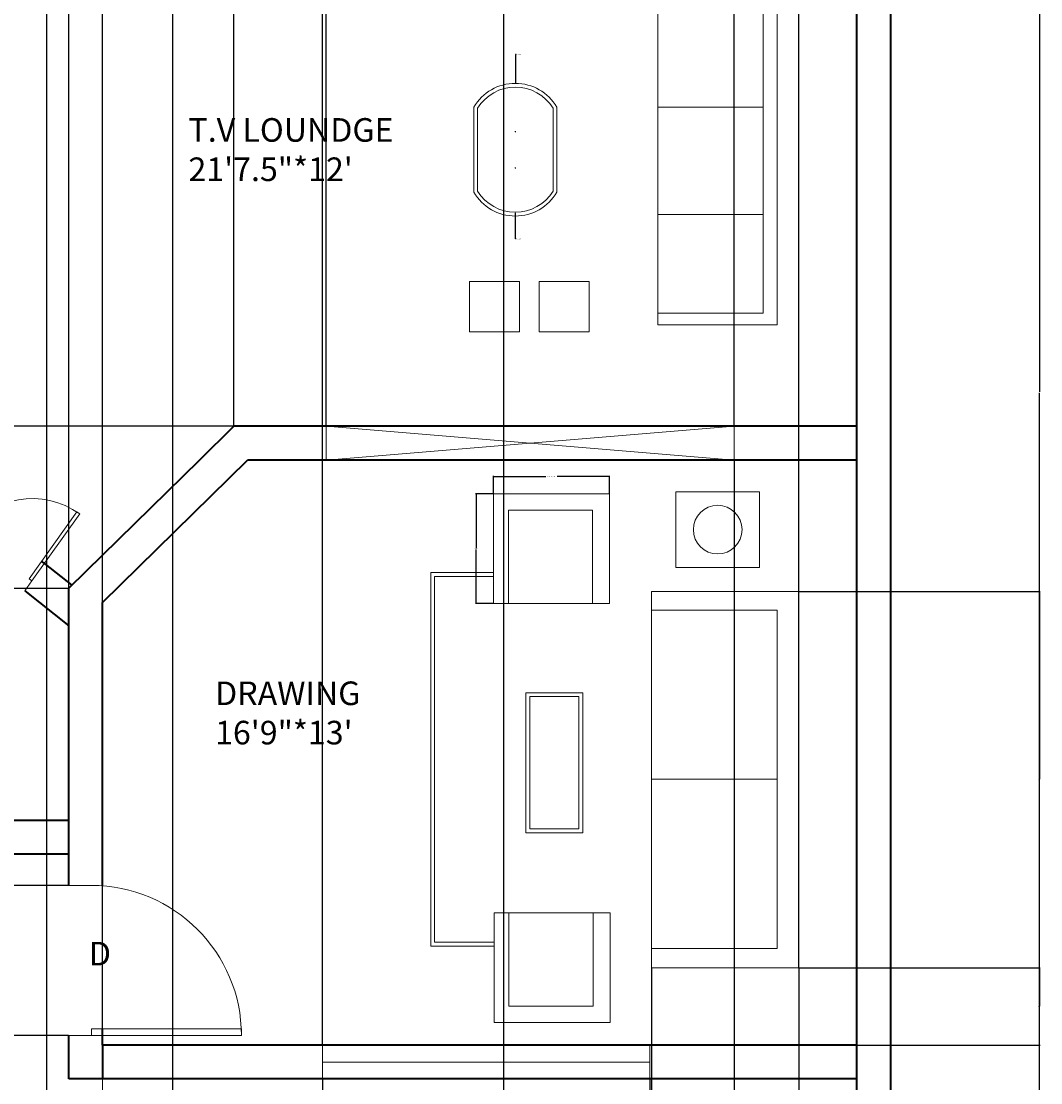
# Model space of a CAD drawing. Units: inches. Extents: x 2284 to 2815, y 1123 to 1948.
# Tile 4 of 6: x 2543 to 2815, y 1358 to 1641. Entities that reach past the tile are written whole.
import ezdxf

# ---------------------------------------------------------------- set-up
doc = ezdxf.new("R2010")
doc.units = ezdxf.units.IN
for name, color, linetype, lineweight in [('A-ANNO-DIMS', 2, 'Continuous', 18), ('A-AREA-IDEN', 30, 'Continuous', 18), ('A-WALL-PATT', 140, 'Continuous', 13), ('C-SITE-PVMT', 7, 'Continuous', 18), ('C-SITE-WALL', 7, 'Continuous', 35), ('DOOR', 190, 'Continuous', 18), ('FUR', 10, 'Continuous', 18), ('TEXT', 30, 'Continuous', 18), ('WALL', 7, 'Continuous', 35), ('WIND', 210, 'Continuous', 18)]:
    doc.layers.add(name, color=color, linetype=linetype, lineweight=lineweight)
doc.styles.get("Standard").update_dxf_attribs({"font": 'arial.ttf'})
doc.dimstyles.get("Standard").update_dxf_attribs({"dimtxt": 0.18, "dimasz": 0.18, "dimexe": 0.18, "dimexo": 0.0625, "dimgap": 0.09, "dimtad": 0, "dimtih": 1, "dimtoh": 1, "dimdec": 4, "dimzin": 0, "dimdsep": 46, "dimtxsty": 'Standard', "dimcen": 0.09, "dimadec": 0, "dimazin": 0, "dimtfac": 1, "dimtdec": 4, "dimtofl": 0, "dimtmove": 0, "dimatfit": 3, "dimfxl": 1, "dimtolj": 1, "dimtzin": 0, "dimarcsym": 0})

# ---------------------------------------------------------------- blocks, each defined once
blk = doc.blocks.new('*U2')
for p, q in [((0, 0), (0, -6)), ((40, 0), (40, -6))]:
    blk.add_line(p, q)
blk.add_lwpolyline([(0, 0), (0, 40), (1.75, 40), (1.75, 0)], close=True)
blk.add_arc((0, 0), 40, 0, 90)
blk = doc.blocks.new('LOUNGE-CHAIR')
for p, q in [((3.98, 0), (3.98, 24.94)), ((3.98, 24.94), (26.41, 24.94)), ((26.41, 24.94), (26.41, 0))]:
    blk.add_line(p, q)
blk.add_lwpolyline([(30.95, 0), (0, 0), (0, 29.22), (30.95, 29.22)], close=True)
blk = doc.blocks.new('*D18')
at = {"layer": 'A-ANNO-DIMS', "color": 0, "lineweight": -2, "transparency": 16777216}
for p, q in [((2668.74, 1515.42), (2668.74, 1520.18)), ((2668.92, 1520), (2682.69, 1520)), ((2699.5, 1520), (2685.73, 1520)), ((2699.68, 1515.42), (2699.68, 1520.18))]:
    blk.add_line(p, q, dxfattribs=at)
at = {"layer": 'A-ANNO-DIMS', "color": 0, "transparency": 16777216}
for points in [[(2668.92, 1520.03), (2668.92, 1519.97), (2668.74, 1520)], [(2699.5, 1520.03), (2699.5, 1519.97), (2699.68, 1520)]]:
    blk.add_solid(points, dxfattribs=at)
at = {"layer": 'Defpoints', "color": 0, "transparency": 16777216}
for p in [(2699.68, 1520), (2668.74, 1515.36), (2699.68, 1515.36)]:
    blk.add_point(p, dxfattribs=at)
at = {"layer": 'A-ANNO-DIMS', "color": 0, "transparency": 16777216, "insert": (2684.21, 1520), "char_height": 0.18, "attachment_point": 5}
blk.add_mtext('\\A1;LOUNGE CHAIR 31 TYP.', dxfattribs=at)
blk = doc.blocks.new('*D19')
at = {"layer": 'A-ANNO-DIMS', "color": 0, "lineweight": -2, "transparency": 16777216}
for p, q in [((2668.67, 1515.36), (2663.91, 1515.36)), ((2664.09, 1515.18), (2664.09, 1500.93)), ((2664.09, 1486.32), (2664.09, 1500.57)), ((2668.67, 1486.14), (2663.91, 1486.14))]:
    blk.add_line(p, q, dxfattribs=at)
at = {"layer": 'A-ANNO-DIMS', "color": 0, "transparency": 16777216}
for points in [[(2664.06, 1515.18), (2664.12, 1515.18), (2664.09, 1515.36)], [(2664.06, 1486.32), (2664.12, 1486.32), (2664.09, 1486.14)]]:
    blk.add_solid(points, dxfattribs=at)
at = {"layer": 'Defpoints', "color": 0, "transparency": 16777216}
for p in [(2664.09, 1515.36), (2668.74, 1515.36), (2668.74, 1486.14)]:
    blk.add_point(p, dxfattribs=at)
at = {"layer": 'A-ANNO-DIMS', "color": 0, "transparency": 16777216, "insert": (2664.09, 1500.75), "char_height": 0.18, "attachment_point": 5}
blk.add_mtext('\\A1;29 TYP.', dxfattribs=at)
blk = doc.blocks.new('*D21')
at = {"layer": 'A-ANNO-DIMS', "color": 0, "lineweight": -2, "transparency": 16777216}
for p, q in [((2774.62, 1908.4), (2814.43, 1908.4)), ((2814.25, 1908.22), (2814.25, 1542.59)), ((2814.25, 1176.58), (2814.25, 1542.22)), ((2774.62, 1176.4), (2814.43, 1176.4))]:
    blk.add_line(p, q, dxfattribs=at)
at = {"layer": 'A-ANNO-DIMS', "color": 0, "transparency": 16777216}
for points in [[(2814.22, 1908.22), (2814.28, 1908.22), (2814.25, 1908.4)], [(2814.22, 1176.58), (2814.28, 1176.58), (2814.25, 1176.4)]]:
    blk.add_solid(points, dxfattribs=at)
at = {"layer": 'Defpoints', "color": 0, "transparency": 16777216}
for p in [(2774.55, 1908.4), (2814.25, 1908.4), (2774.55, 1176.4)]:
    blk.add_point(p, dxfattribs=at)
at = {"layer": 'A-ANNO-DIMS', "color": 0, "transparency": 16777216, "insert": (2814.25, 1542.4), "char_height": 0.18, "attachment_point": 5}
blk.add_mtext('\\A1;732', dxfattribs=at)
blk = doc.blocks.new('*D42')
at = {"layer": 'A-ANNO-DIMS', "color": 0, "lineweight": -2, "transparency": 16777216}
for p, q in [((2623.18, 1359.34), (2623.18, 1136.52)), ((2710.41, 1359.34), (2710.41, 1136.52)), ((2623.36, 1136.7), (2666.4, 1136.7)), ((2710.23, 1136.7), (2667.19, 1136.7))]:
    blk.add_line(p, q, dxfattribs=at)
at = {"layer": 'A-ANNO-DIMS', "color": 0, "transparency": 16777216}
for points in [[(2623.36, 1136.73), (2623.36, 1136.67), (2623.18, 1136.7)], [(2710.23, 1136.73), (2710.23, 1136.67), (2710.41, 1136.7)]]:
    blk.add_solid(points, dxfattribs=at)
at = {"layer": 'Defpoints', "color": 0, "transparency": 16777216}
for p in [(2623.18, 1359.4), (2710.41, 1359.4), (2710.41, 1136.7)]:
    blk.add_point(p, dxfattribs=at)
at = {"layer": 'A-ANNO-DIMS', "color": 0, "transparency": 16777216, "insert": (2666.79, 1136.7), "char_height": 0.18, "attachment_point": 5}
blk.add_mtext('\\A1;87.23', dxfattribs=at)
blk = doc.blocks.new('*D43')
at = {"layer": 'A-ANNO-DIMS', "color": 0, "lineweight": -2, "transparency": 16777216}
for p, q in [((2564.55, 1368.47), (2564.55, 1948.28)), ((2564.73, 1948.1), (2593.47, 1948.1)), ((2623, 1948.1), (2594.26, 1948.1)), ((2623.18, 1368.47), (2623.18, 1948.28))]:
    blk.add_line(p, q, dxfattribs=at)
at = {"layer": 'A-ANNO-DIMS', "color": 0, "transparency": 16777216}
for points in [[(2564.73, 1948.13), (2564.73, 1948.07), (2564.55, 1948.1)], [(2623, 1948.13), (2623, 1948.07), (2623.18, 1948.1)]]:
    blk.add_solid(points, dxfattribs=at)
at = {"layer": 'Defpoints', "color": 0, "transparency": 16777216}
for p in [(2623.18, 1948.1), (2564.55, 1368.4), (2623.18, 1368.4)]:
    blk.add_point(p, dxfattribs=at)
at = {"layer": 'A-ANNO-DIMS', "color": 0, "transparency": 16777216, "insert": (2593.87, 1948.1), "char_height": 0.18, "attachment_point": 5}
blk.add_mtext('\\A1;58.62', dxfattribs=at)
blk = doc.blocks.new('*D44')
at = {"layer": 'A-ANNO-DIMS', "color": 0, "lineweight": -2, "transparency": 16777216}
for p, q in [((2583.19, 1836.34), (2583.19, 1136.52)), ((2671.4, 1836.34), (2671.4, 1136.52)), ((2583.37, 1136.7), (2626.92, 1136.7)), ((2671.22, 1136.7), (2627.67, 1136.7))]:
    blk.add_line(p, q, dxfattribs=at)
at = {"layer": 'A-ANNO-DIMS', "color": 0, "transparency": 16777216}
for points in [[(2583.37, 1136.73), (2583.37, 1136.67), (2583.19, 1136.7)], [(2671.22, 1136.73), (2671.22, 1136.67), (2671.4, 1136.7)]]:
    blk.add_solid(points, dxfattribs=at)
at = {"layer": 'Defpoints', "color": 0, "transparency": 16777216}
for p in [(2583.19, 1836.4), (2671.4, 1836.4), (2671.4, 1136.7)]:
    blk.add_point(p, dxfattribs=at)
at = {"layer": 'A-ANNO-DIMS', "color": 0, "transparency": 16777216, "insert": (2627.29, 1136.7), "char_height": 0.18, "attachment_point": 5}
blk.add_mtext('\\A1;88.21', dxfattribs=at)
blk = doc.blocks.new('*D45')
at = {"layer": 'A-ANNO-DIMS', "color": 0, "lineweight": -2, "transparency": 16777216}
for p, q in [((2549.55, 1836.34), (2549.55, 1136.52)), ((2583.19, 1836.34), (2583.19, 1136.52)), ((2549.73, 1136.7), (2565.91, 1136.7)), ((2583.01, 1136.7), (2566.84, 1136.7))]:
    blk.add_line(p, q, dxfattribs=at)
at = {"layer": 'A-ANNO-DIMS', "color": 0, "transparency": 16777216}
for points in [[(2549.73, 1136.73), (2549.73, 1136.67), (2549.55, 1136.7)], [(2583.01, 1136.73), (2583.01, 1136.67), (2583.19, 1136.7)]]:
    blk.add_solid(points, dxfattribs=at)
at = {"layer": 'Defpoints', "color": 0, "transparency": 16777216}
for p in [(2549.55, 1836.4), (2583.19, 1836.4), (2583.19, 1136.7)]:
    blk.add_point(p, dxfattribs=at)
at = {"layer": 'A-ANNO-DIMS', "color": 0, "transparency": 16777216, "insert": (2566.37, 1136.7), "char_height": 0.18, "attachment_point": 5}
blk.add_mtext('\\A1;33.635', dxfattribs=at)
blk = doc.blocks.new('*D47')
at = {"layer": 'A-ANNO-DIMS', "color": 0, "lineweight": -2, "transparency": 16777216}
for p, q in [((2555.49, 1410.98), (2284.67, 1410.98)), ((2284.85, 1410.8), (2284.85, 1391.17)), ((2284.85, 1371.16), (2284.85, 1390.8)), ((2555.49, 1370.98), (2284.67, 1370.98))]:
    blk.add_line(p, q, dxfattribs=at)
at = {"layer": 'A-ANNO-DIMS', "color": 0, "transparency": 16777216}
for points in [[(2284.82, 1410.8), (2284.88, 1410.8), (2284.85, 1410.98)], [(2284.82, 1371.16), (2284.88, 1371.16), (2284.85, 1370.98)]]:
    blk.add_solid(points, dxfattribs=at)
at = {"layer": 'Defpoints', "color": 0, "transparency": 16777216}
for p in [(2284.85, 1410.98), (2555.55, 1410.98), (2555.55, 1370.98)]:
    blk.add_point(p, dxfattribs=at)
at = {"layer": 'A-ANNO-DIMS', "color": 0, "transparency": 16777216, "insert": (2284.85, 1390.98), "char_height": 0.18, "attachment_point": 5}
blk.add_mtext('\\A1;40', dxfattribs=at)
blk = doc.blocks.new('*D48')
at = {"layer": 'A-ANNO-DIMS', "color": 0, "lineweight": -2, "transparency": 16777216}
for p, q in [((2624.18, 1533.47), (2624.18, 1948.28)), ((2624.36, 1948.1), (2678.14, 1948.1)), ((2732.7, 1948.1), (2678.91, 1948.1)), ((2732.88, 1533.47), (2732.88, 1948.28))]:
    blk.add_line(p, q, dxfattribs=at)
at = {"layer": 'A-ANNO-DIMS', "color": 0, "transparency": 16777216}
for points in [[(2624.36, 1948.13), (2624.36, 1948.07), (2624.18, 1948.1)], [(2732.7, 1948.13), (2732.7, 1948.07), (2732.88, 1948.1)]]:
    blk.add_solid(points, dxfattribs=at)
at = {"layer": 'Defpoints', "color": 0, "transparency": 16777216}
for p in [(2732.88, 1948.1), (2624.18, 1533.4), (2732.88, 1533.4)]:
    blk.add_point(p, dxfattribs=at)
at = {"layer": 'A-ANNO-DIMS', "color": 0, "transparency": 16777216, "insert": (2678.53, 1948.1), "char_height": 0.18, "attachment_point": 5}
blk.add_mtext('\\A1;108.7', dxfattribs=at)
blk = doc.blocks.new('*D49')
at = {"layer": 'A-ANNO-DIMS', "color": 0, "lineweight": -2, "transparency": 16777216}
for p, q in [((2732.88, 1524.34), (2732.88, 1136.52)), ((2765.55, 1524.34), (2765.55, 1136.52)), ((2733.06, 1136.7), (2748.82, 1136.7)), ((2765.37, 1136.7), (2749.61, 1136.7))]:
    blk.add_line(p, q, dxfattribs=at)
at = {"layer": 'A-ANNO-DIMS', "color": 0, "transparency": 16777216}
for points in [[(2733.06, 1136.73), (2733.06, 1136.67), (2732.88, 1136.7)], [(2765.37, 1136.73), (2765.37, 1136.67), (2765.55, 1136.7)]]:
    blk.add_solid(points, dxfattribs=at)
at = {"layer": 'Defpoints', "color": 0, "transparency": 16777216}
for p in [(2732.88, 1524.4), (2765.55, 1524.4), (2765.55, 1136.7)]:
    blk.add_point(p, dxfattribs=at)
at = {"layer": 'A-ANNO-DIMS', "color": 0, "transparency": 16777216, "insert": (2749.21, 1136.7), "char_height": 0.18, "attachment_point": 5}
blk.add_mtext('\\A1;32.68', dxfattribs=at)
blk = doc.blocks.new('*D50')
at = {"layer": 'A-ANNO-DIMS', "color": 0, "lineweight": -2, "transparency": 16777216}
for p, q in [((2750.17, 1489.33), (2814.43, 1489.33)), ((2814.25, 1489.15), (2814.25, 1439.34)), ((2814.25, 1389.18), (2814.25, 1438.98)), ((2750.17, 1389), (2814.43, 1389))]:
    blk.add_line(p, q, dxfattribs=at)
at = {"layer": 'A-ANNO-DIMS', "color": 0, "transparency": 16777216}
for points in [[(2814.22, 1489.15), (2814.28, 1489.15), (2814.25, 1489.33)], [(2814.22, 1389.18), (2814.28, 1389.18), (2814.25, 1389)]]:
    blk.add_solid(points, dxfattribs=at)
at = {"layer": 'Defpoints', "color": 0, "transparency": 16777216}
for p in [(2750.11, 1489.33), (2814.25, 1489.33), (2750.11, 1389)]:
    blk.add_point(p, dxfattribs=at)
at = {"layer": 'A-ANNO-DIMS', "color": 0, "transparency": 16777216, "insert": (2814.25, 1439.16), "char_height": 0.18, "attachment_point": 5}
blk.add_mtext('\\A1;100.33', dxfattribs=at)
blk = doc.blocks.new('*D51')
at = {"layer": 'A-ANNO-DIMS', "color": 0, "lineweight": -2, "transparency": 16777216}
for p, q in [((2710.87, 1388.93), (2710.87, 1136.52)), ((2750.11, 1388.93), (2750.11, 1136.52)), ((2711.05, 1136.7), (2730.03, 1136.7)), ((2749.93, 1136.7), (2730.95, 1136.7))]:
    blk.add_line(p, q, dxfattribs=at)
at = {"layer": 'A-ANNO-DIMS', "color": 0, "transparency": 16777216}
for points in [[(2711.05, 1136.73), (2711.05, 1136.67), (2710.87, 1136.7)], [(2749.93, 1136.73), (2749.93, 1136.67), (2750.11, 1136.7)]]:
    blk.add_solid(points, dxfattribs=at)
at = {"layer": 'Defpoints', "color": 0, "transparency": 16777216}
for p in [(2710.87, 1389), (2750.11, 1389), (2750.11, 1136.7)]:
    blk.add_point(p, dxfattribs=at)
at = {"layer": 'A-ANNO-DIMS', "color": 0, "transparency": 16777216, "insert": (2730.49, 1136.7), "char_height": 0.18, "attachment_point": 5}
blk.add_mtext('\\A1;39.234', dxfattribs=at)
blk = doc.blocks.new('*D52')
at = {"layer": 'A-ANNO-DIMS', "color": 0, "lineweight": -2, "transparency": 16777216}
for p, q in [((2750.11, 1389.06), (2750.11, 1948.28)), ((2750.29, 1948.1), (2757.37, 1948.1)), ((2765.37, 1948.1), (2758.29, 1948.1)), ((2765.55, 1368.47), (2765.55, 1948.28))]:
    blk.add_line(p, q, dxfattribs=at)
at = {"layer": 'A-ANNO-DIMS', "color": 0, "transparency": 16777216}
for points in [[(2750.29, 1948.13), (2750.29, 1948.07), (2750.11, 1948.1)], [(2765.37, 1948.13), (2765.37, 1948.07), (2765.55, 1948.1)]]:
    blk.add_solid(points, dxfattribs=at)
at = {"layer": 'Defpoints', "color": 0, "transparency": 16777216}
for p in [(2765.55, 1948.1), (2750.11, 1389), (2765.55, 1368.4)]:
    blk.add_point(p, dxfattribs=at)
at = {"layer": 'A-ANNO-DIMS', "color": 0, "transparency": 16777216, "insert": (2757.83, 1948.1), "char_height": 0.18, "attachment_point": 5}
blk.add_mtext('\\A1;15.448', dxfattribs=at)
blk = doc.blocks.new('*D53')
at = {"layer": 'A-ANNO-DIMS', "color": 0, "lineweight": -2, "transparency": 16777216}
for p, q in [((2750.17, 1389), (2814.43, 1389)), ((2814.25, 1388.82), (2814.25, 1378.88)), ((2814.25, 1368.58), (2814.25, 1378.52)), ((2765.62, 1368.4), (2814.43, 1368.4))]:
    blk.add_line(p, q, dxfattribs=at)
at = {"layer": 'A-ANNO-DIMS', "color": 0, "transparency": 16777216}
for points in [[(2814.22, 1388.82), (2814.28, 1388.82), (2814.25, 1389)], [(2814.22, 1368.58), (2814.28, 1368.58), (2814.25, 1368.4)]]:
    blk.add_solid(points, dxfattribs=at)
at = {"layer": 'Defpoints', "color": 0, "transparency": 16777216}
for p in [(2750.11, 1389), (2814.25, 1389), (2765.55, 1368.4)]:
    blk.add_point(p, dxfattribs=at)
at = {"layer": 'A-ANNO-DIMS', "color": 0, "transparency": 16777216, "insert": (2814.25, 1378.7), "char_height": 0.18, "attachment_point": 5}
blk.add_mtext('\\A1;20.59', dxfattribs=at)
blk = doc.blocks.new('*D54')
at = {"layer": 'A-ANNO-DIMS', "color": 0, "lineweight": -2, "transparency": 16777216}
for p, q in [((2555.55, 1490.27), (2555.55, 1948.28)), ((2555.73, 1948.1), (2577.07, 1948.1)), ((2599.35, 1948.1), (2578.01, 1948.1)), ((2599.53, 1533.47), (2599.53, 1948.28))]:
    blk.add_line(p, q, dxfattribs=at)
at = {"layer": 'A-ANNO-DIMS', "color": 0, "transparency": 16777216}
for points in [[(2555.73, 1948.13), (2555.73, 1948.07), (2555.55, 1948.1)], [(2599.35, 1948.13), (2599.35, 1948.07), (2599.53, 1948.1)]]:
    blk.add_solid(points, dxfattribs=at)
at = {"layer": 'Defpoints', "color": 0, "transparency": 16777216}
for p in [(2599.53, 1948.1), (2599.53, 1533.4), (2555.55, 1490.2)]:
    blk.add_point(p, dxfattribs=at)
at = {"layer": 'A-ANNO-DIMS', "color": 0, "transparency": 16777216, "insert": (2577.54, 1948.1), "char_height": 0.18, "attachment_point": 5}
blk.add_mtext('\\A1;43.975', dxfattribs=at)
blk = doc.blocks.new('*D55')
at = {"layer": 'A-ANNO-DIMS', "color": 0, "lineweight": -2, "transparency": 16777216}
for p, q in [((2599.47, 1533.4), (2284.67, 1533.4)), ((2284.85, 1533.22), (2284.85, 1511.99)), ((2284.85, 1490.38), (2284.85, 1511.62)), ((2555.49, 1490.2), (2284.67, 1490.2))]:
    blk.add_line(p, q, dxfattribs=at)
at = {"layer": 'A-ANNO-DIMS', "color": 0, "transparency": 16777216}
for points in [[(2284.82, 1533.22), (2284.88, 1533.22), (2284.85, 1533.4)], [(2284.82, 1490.38), (2284.88, 1490.38), (2284.85, 1490.2)]]:
    blk.add_solid(points, dxfattribs=at)
at = {"layer": 'Defpoints', "color": 0, "transparency": 16777216}
for p in [(2284.85, 1533.4), (2599.53, 1533.4), (2555.55, 1490.2)]:
    blk.add_point(p, dxfattribs=at)
at = {"layer": 'A-ANNO-DIMS', "color": 0, "transparency": 16777216, "insert": (2284.85, 1511.8), "char_height": 0.18, "attachment_point": 5}
blk.add_mtext('\\A1;43.2', dxfattribs=at)
blk = doc.blocks.new('*D69')
at = {"layer": 'A-ANNO-DIMS', "color": 0, "lineweight": -2, "transparency": 16777216}
for p, q in [((2674.75, 1632.55), (2674.57, 1632.55)), ((2674.57, 1632.55), (2674.57, 1625.02)), ((2674.48, 1611.99), (2674.66, 1611.99)), ((2674.57, 1611.9), (2674.57, 1612.08))]:
    blk.add_line(p, q, dxfattribs=at)
at = {"layer": 'A-ANNO-DIMS', "color": 0, "transparency": 16777216}
blk.add_solid([(2674.54, 1625.02), (2674.6, 1625.02), (2674.57, 1624.84)], dxfattribs=at)
at = {"layer": 'Defpoints', "color": 0, "transparency": 16777216}
for p in [(2674.57, 1624.84), (2674.57, 1611.99)]:
    blk.add_point(p, dxfattribs=at)
at = {"layer": 'A-ANNO-DIMS', "color": 0, "transparency": 16777216, "insert": (2675.5, 1632.55), "char_height": 0.18, "attachment_point": 5}
blk.add_mtext('\\A1;2X R12.848', dxfattribs=at)
blk = doc.blocks.new('*D70')
at = {"layer": 'A-ANNO-DIMS', "color": 0, "lineweight": -2, "transparency": 16777216}
for p, q in [((2674.48, 1602.32), (2674.66, 1602.32)), ((2674.57, 1602.23), (2674.57, 1602.41)), ((2674.57, 1583.36), (2674.57, 1590.29)), ((2674.75, 1583.36), (2674.57, 1583.36))]:
    blk.add_line(p, q, dxfattribs=at)
at = {"layer": 'A-ANNO-DIMS', "color": 0, "transparency": 16777216}
blk.add_solid([(2674.6, 1590.29), (2674.54, 1590.29), (2674.57, 1590.47)], dxfattribs=at)
at = {"layer": 'Defpoints', "color": 0, "transparency": 16777216}
for p in [(2674.57, 1602.32), (2674.57, 1590.47)]:
    blk.add_point(p, dxfattribs=at)
at = {"layer": 'A-ANNO-DIMS', "color": 0, "transparency": 16777216, "insert": (2675.5, 1583.36), "char_height": 0.18, "attachment_point": 5}
blk.add_mtext('\\A1;2X R11.848', dxfattribs=at)

msp = doc.modelspace()

# ---------------------------------------------------------------- hatches: boundary and pattern name
at = {"layer": 'A-WALL-PATT'}
h = msp.add_hatch(dxfattribs=at)
h.set_pattern_fill('AR-SAND', color=256, scale=8.5)
h.paths.add_polyline_path([(2339.554, 1899.404), (2375.554, 1899.404), (2765.554, 1899.404), (2765.554, 1185.404), (2549.3222, 1185.404), (2549.3222, 1176.404), (2774.554, 1176.404), (2774.554, 1908.404), (2330.554, 1908.404), (2330.554, 1176.404), (2349.4276, 1176.404), (2349.4276, 1185.404), (2339.554, 1185.404)])
h.paths.add_polyline_path([(2710.054, 1899.404), (2701.054, 1899.404), (2701.054, 1889.8374), (2710.054, 1889.8374)], flags=17)
h = msp.add_hatch(dxfattribs=at)
h.set_pattern_fill('AR-SAND', color=256, scale=8.5)
h.paths.add_polyline_path([(2549.554, 1863.404), (2375.554, 1863.404), (2375.554, 1840.6021), (2384.554, 1840.6021), (2384.554, 1854.404), (2480.554, 1854.404), (2549.554, 1854.404)])
h.paths.add_polyline_path([(2384.554, 1795.904), (2384.554, 1809.1528), (2375.554, 1809.1528), (2375.554, 1758.7416), (2384.554, 1758.7416)])
h.paths.add_polyline_path([(2549.554, 1836.404), (2549.554, 1854.404), (2540.554, 1854.404), (2540.554, 1800.404), (2485.054, 1800.404), (2485.054, 1802.7347), (2480.554, 1802.7347), (2480.554, 1800.404), (2384.554, 1800.404), (2384.554, 1795.904), (2485.054, 1795.904), (2540.554, 1795.904), (2540.554, 1678.5102), (2543.2164, 1676.3784), (2547.9, 1672.6283), (2549.554, 1677.404), (2549.554, 1795.904)])
h.paths.add_polyline_path([(2452.31, 1803.9815), (2480.7795, 1803.9815), (2480.7795, 1802.7347), (2452.2828, 1802.7347), (2452.2828, 1803.9815), (2452.31, 1803.9815, -0.39915744), (2480.554, 1831.2306), (2480.554, 1854.404), (2540.554, 1854.404), (2485.054, 1837.4988), (2485.054, 1831.2315), (2480.7795, 1831.2315, 0.40145271)], flags=17)
h.paths.add_polyline_path([(2583.189, 1845.404), (2549.554, 1845.404), (2549.554, 1836.404), (2583.189, 1836.404)])
h.paths.add_polyline_path([(2710.054, 1858.3882), (2701.054, 1858.3882), (2701.054, 1845.404), (2671.4007, 1845.404), (2671.4007, 1836.404), (2710.054, 1836.404)])
h.paths.add_polyline_path([(2710.054, 1836.404), (2705.554, 1836.404), (2705.554, 1774.904), (2710.054, 1774.904), (2710.054, 1779.404)])
h.paths.add_polyline_path([(2765.554, 1779.404), (2737.9116, 1779.404, -0.00645116), (2737.9201, 1778.7436), (2737.9201, 1774.904), (2765.554, 1774.904)])
h.paths.add_polyline_path([(2712.3231, 1778.7436), (2712.3231, 1779.404), (2710.054, 1779.404), (2710.054, 1774.904), (2712.3231, 1774.904)])
h.paths.add_polyline_path([(2710.054, 1774.904), (2705.554, 1774.904), (2705.554, 1769.4647), (2710.054, 1769.4647)])
h.paths.add_polyline_path([(2710.054, 1702.7233), (2705.554, 1702.7233), (2705.554, 1686.404), (2592.0733, 1686.404, -0.01876983), (2592.186, 1683.404), (2592.186, 1677.404), (2705.554, 1677.404), (2765.554, 1677.404), (2765.554, 1686.404), (2710.054, 1686.404)])
h.paths.add_polyline_path([(2384.554, 1641.404), (2375.554, 1641.404), (2375.554, 1637.3708), (2381.554, 1637.3708), (2384.554, 1637.3708)])
h.paths.add_polyline_path([(2384.554, 1678.0573), (2375.554, 1678.0573), (2375.554, 1641.404), (2384.554, 1641.404), (2522.8991, 1641.404), (2518.2155, 1645.1541, -0.00736412), (2517.3067, 1645.904), (2384.554, 1645.904)])
h.paths.add_polyline_path([(2384.554, 1597.4834, -0.01876983), (2381.554, 1597.3708), (2375.554, 1597.3708), (2375.554, 1591.564), (2384.554, 1591.564)])
h.paths.add_polyline_path([(2384.554, 1533.404), (2384.554, 1538.4896), (2375.554, 1538.4896), (2375.554, 1524.404), (2384.554, 1524.404)])
h.paths.add_polyline_path([(2506.054, 1533.404), (2506.054, 1598.7748), (2500.054, 1598.7748, -0.01876983), (2497.054, 1598.8874), (2497.054, 1533.404), (2384.554, 1533.404), (2384.554, 1524.404), (2497.054, 1524.404), (2506.054, 1524.404)])
h.paths.add_polyline_path([(2473.054, 1446.985), (2468.9674, 1446.985, -0.00379375), (2468.554, 1446.9881), (2468.554, 1428.404), (2473.054, 1428.404)])
h.paths.add_polyline_path([(2384.554, 1524.404), (2375.554, 1524.404), (2375.554, 1468.4232), (2384.554, 1468.4232)])
h.paths.add_polyline_path([(2473.054, 1480.904), (2384.554, 1480.904), (2384.554, 1476.404), (2468.554, 1476.404), (2468.554, 1474.2289), (2468.9674, 1474.2289), (2473.054, 1474.2289)])
h.paths.add_polyline_path([(2555.554, 1428.404), (2546.554, 1428.404), (2539.1317, 1428.404), (2539.1317, 1422.885), (2539.1317, 1419.404), (2546.554, 1419.404), (2555.554, 1419.404)])
h.paths.add_polyline_path([(2564.554, 1368.404), (2564.554, 1370.9838), (2561.554, 1370.9838), (2555.554, 1370.9838), (2555.554, 1359.404), (2564.554, 1359.404)])
h.paths.add_polyline_path([(2623.1768, 1368.404), (2564.554, 1368.404), (2564.554, 1359.404), (2623.1768, 1359.404)])
h.paths.add_polyline_path([(2492.7181, 1422.885), (2492.7181, 1428.404), (2384.554, 1428.404), (2384.554, 1440.6426), (2375.554, 1440.6426), (2375.554, 1419.404), (2492.7181, 1419.404)])
h.paths.add_polyline_path([(2765.554, 1368.404), (2710.406, 1368.404), (2710.406, 1359.404), (2765.554, 1359.404)])
h.paths.add_polyline_path([(2765.554, 1533.404), (2732.876, 1533.404), (2732.876, 1524.404), (2765.554, 1524.404)])
h.paths.add_polyline_path([(2624.1792, 1533.404), (2599.5288, 1533.404), (2590.3672, 1524.404), (2564.554, 1499.046), (2555.554, 1490.2048), (2555.554, 1410.9838), (2561.554, 1410.9838, -0.01876983), (2564.554, 1410.8712), (2564.554, 1486.4298), (2603.2099, 1524.404), (2624.1792, 1524.404)])
h.paths.add_polyline_path([(2555.554, 1490.2048), (2556.4043, 1491.0401), (2549.047, 1496.8538), (2545.7227, 1492.1958), (2543.8126, 1489.5193), (2555.554, 1480.2413)])
h.paths.add_polyline_path([(2514.6892, 1524.0031), (2506.054, 1530.8266), (2506.054, 1524.404), (2499.6656, 1524.404), (2500.474, 1523.7652), (2509.4548, 1516.6686), (2511.3649, 1519.3451)])
h.paths.add_polyline_path([(2365.9834, 1447.3726), (2374.9891, 1447.3726), (2374.9891, 1460.3342), (2365.9834, 1460.3342)], flags=9)
h.paths.add_polyline_path([(2366.9945, 1818.7713), (2376.0002, 1818.7713), (2376.0002, 1831.7328), (2366.9945, 1831.7328)], flags=9)
h.paths.add_polyline_path([(2363.2989, 1558.2059), (2374.7373, 1558.2059), (2374.7373, 1571.1674), (2363.2989, 1571.1674)], flags=9)
h.paths.add_polyline_path([(2364.8137, 1707.1012), (2376.2521, 1707.1012), (2376.2521, 1720.0627), (2364.8137, 1720.0627)], flags=9)
h.paths.add_polyline_path([(2460.3189, 1455.9932), (2469.8094, 1455.9932), (2469.8094, 1468.9547), (2460.3189, 1468.9547)], flags=9)
h.paths.add_polyline_path([(2558.6325, 1386.2225), (2568.1231, 1386.2225), (2568.1231, 1399.184), (2558.6325, 1399.184)], flags=9)
h.paths.add_polyline_path([(2378.5629, 1611.6816), (2388.0534, 1611.6816), (2388.0534, 1624.6431), (2378.5629, 1624.6431)], flags=9)
h.paths.add_polyline_path([(2490.2277, 1613.2326), (2499.7182, 1613.2326), (2499.7182, 1626.1941), (2490.2277, 1626.1941)], flags=9)
h.paths.add_polyline_path([(2522.9652, 1656.7942), (2532.4557, 1656.7942), (2532.4557, 1669.7557), (2522.9652, 1669.7557)], flags=9)
h.paths.add_polyline_path([(2567.5462, 1677.3031), (2577.0367, 1677.3031), (2577.0367, 1690.2646), (2567.5462, 1690.2646)], flags=9)
h.paths.add_polyline_path([(2363.196, 1676.9136), (2363.196, 1756.4461), (2350.2345, 1756.4461), (2350.2345, 1676.9136)], flags=9)
h.paths.add_polyline_path([(2515.5569, 1505.5998), (2535.7182, 1488.4964), (2539.8301, 1493.3434), (2519.6687, 1510.4468)], flags=9)
h.paths.add_polyline_path([(2503.6006, 1414.6146), (2530.0393, 1414.6146), (2530.0393, 1420.9707), (2503.6006, 1420.9707)], flags=9)
h.paths.add_polyline_path([(2391.2946, 1877.326), (2470.827, 1877.326), (2470.827, 1890.2876), (2391.2946, 1890.2876)], flags=9)
h.paths.add_polyline_path([(2580.3233, 1794.4386), (2629.1831, 1794.4386), (2629.1831, 1817.9089), (2580.3233, 1817.9089)], flags=9)
h.paths.add_polyline_path([(2585.6043, 1595.2228), (2648.3653, 1595.2228), (2648.3653, 1618.6931), (2585.6043, 1618.6931)], flags=9)
h.paths.add_polyline_path([(2591.9981, 1445.0189), (2637.889, 1445.0189), (2637.889, 1468.4892), (2591.9981, 1468.4892)], flags=9)
h.paths.add_polyline_path([(2459.0727, 1376.5795), (2515.4624, 1376.5795), (2515.4624, 1400.0498), (2459.0727, 1400.0498)], flags=9)
h.paths.add_polyline_path([(2481.8769, 1451.6363), (2543.2049, 1451.6363), (2543.2049, 1475.1066), (2481.8769, 1475.1066)], flags=9)
h.paths.add_polyline_path([(2470.0329, 1495.943), (2485.3842, 1495.943), (2485.3842, 1508.9045), (2470.0329, 1508.9045)], flags=9)
h.paths.add_polyline_path([(2419.5143, 1438.0898), (2446.0938, 1438.0898), (2446.0938, 1461.5344), (2419.5143, 1461.5344)], flags=9)
h.paths.add_polyline_path([(2425.6893, 1570.7133), (2467.4012, 1570.7133), (2467.4012, 1594.1836), (2425.6893, 1594.1836)], flags=25)
h.paths.add_polyline_path([(2428.101, 1758.2973), (2476.9609, 1758.2973), (2476.9609, 1781.7676), (2428.101, 1781.7676)], flags=25)

# ---------------------------------------------------------------- linework, layer by layer
at = {"layer": 'C-SITE-PVMT'}
msp.add_line((2564.554, 1359.404), (2564.554, 1185.404), dxfattribs=at)
at = {"layer": 'C-SITE-WALL'}
for p, q in [((2774.554, 1908.404), (2774.554, 1176.404)), ((2765.554, 1899.404), (2765.554, 1185.404))]:
    msp.add_line(p, q, dxfattribs=at)
at = {"layer": 'FUR'}
for p, q in [((2740.6212, 1563.5556), (2740.6212, 1643.8812)), ((2712.5251, 1618.4665), (2740.6212, 1618.4665)), ((2712.5251, 1589.9141), (2740.6212, 1589.9141)), ((2712.5251, 1563.5556), (2712.5251, 1563.5556)), ((2712.5251, 1563.5556), (2740.6212, 1563.5556)), ((2652.0605, 1394.8191), (2652.0605, 1494.3811)), ((2652.0605, 1494.3811), (2668.7371, 1494.3811)), ((2653.0605, 1395.8191), (2653.0605, 1493.3811)), ((2653.0605, 1493.3811), (2668.7371, 1493.3811)), ((2710.8724, 1484.3921), (2710.8724, 1489.3264)), ((2710.8724, 1489.3264), (2750.1064, 1489.3264)), ((2750.1064, 1489.3264), (2750.1064, 1388.9955)), ((2710.8724, 1439.298), (2744.3448, 1439.298)), ((2710.8724, 1388.9955), (2710.8724, 1405.4432)), ((2668.8886, 1395.8191), (2653.0605, 1395.8191)), ((2668.8886, 1394.8191), (2652.0605, 1394.8191)), ((2750.1064, 1388.9955), (2710.8724, 1388.9955))]:
    msp.add_line(p, q, dxfattribs=at)
for points in [[(2744.3301, 1646.5004), (2712.5251, 1646.5004), (2712.5251, 1560.4509), (2744.3301, 1560.4509)], [(2675.6445, 1572), (2662.3672, 1572), (2662.3672, 1558.628), (2675.6445, 1558.628)], [(2694.2327, 1572), (2680.9554, 1572), (2680.9554, 1558.628), (2694.2327, 1558.628)], [(2717.3295, 1495.7887), (2739.6919, 1495.7887), (2739.6919, 1515.925), (2717.3295, 1515.925)], [(2744.3448, 1484.3921), (2710.8724, 1484.3921), (2710.8724, 1394.2039), (2744.3448, 1394.2039)], [(2692.5318, 1462.3477), (2677.392, 1462.3477), (2677.392, 1425.0466), (2692.5318, 1425.0466)], [(2691.5318, 1461.3477), (2678.392, 1461.3477), (2678.392, 1426.0466), (2691.5318, 1426.0466)]]:
    msp.add_lwpolyline(points, close=True, dxfattribs=at)
for points in [[(2663.5014, 1618.512), (2663.5014, 1595.7959)], [(2664.5014, 1618.2334), (2664.5014, 1596.0745)], [(2684.642, 1596.0745), (2684.642, 1618.2334)], [(2685.642, 1595.7959), (2685.642, 1618.512)]]:
    msp.add_lwpolyline(points, dxfattribs=at)
msp.add_circle((2728.5107, 1505.8569), 6.4878, dxfattribs=at)
for centre, radius, start, end in [((2674.5717, 1611.9904), 12.8485, 30.502749, 149.497251), ((2674.5717, 1611.9904), 11.8485, 31.796555, 148.203445), ((2674.5717, 1602.3176), 12.8485, 210.502749, 329.497251), ((2674.5717, 1602.3176), 11.8485, 211.796555, 328.203445)]:
    msp.add_arc(centre, radius, start, end, dxfattribs=at)
at = {"layer": 'WALL'}
for p, q in [((2765.554, 1677.404), (2765.554, 1533.404)), ((2590.3672, 1524.404), (2599.5288, 1533.404)), ((2765.554, 1533.404), (2599.5288, 1533.404)), ((2564.554, 1486.4298), (2603.2099, 1524.404)), ((2564.554, 1499.046), (2590.3672, 1524.404)), ((2765.554, 1524.404), (2603.2099, 1524.404)), ((2765.554, 1524.404), (2765.554, 1368.404)), ((2549.3522, 1496.6126), (2548.2936, 1497.4491)), ((2564.554, 1499.046), (2555.554, 1490.2048)), ((2556.4043, 1491.0401), (2549.3522, 1496.6126)), ((2543.7723, 1489.5511), (2555.554, 1480.2413)), ((2555.554, 1410.9838), (2555.554, 1490.2048)), ((2564.554, 1410.8712), (2564.554, 1486.4298)), ((2538.1164, 1428.404), (2546.554, 1428.404)), ((2546.554, 1428.404), (2555.554, 1428.404)), ((2539.1317, 1419.404), (2546.554, 1419.404)), ((2546.554, 1419.404), (2555.554, 1419.404)), ((2564.554, 1368.404), (2564.554, 1372.7338)), ((2555.554, 1359.404), (2555.554, 1370.9838)), ((2765.554, 1368.404), (2564.554, 1368.404)), ((2564.554, 1368.404), (2564.554, 1359.404)), ((2765.554, 1359.404), (2555.554, 1359.404))]:
    msp.add_line(p, q, dxfattribs=at)
at = {"layer": 'WIND'}
for p, q in [((2624.1792, 1533.404), (2624.1792, 1524.404)), ((2624.1792, 1524.404), (2732.876, 1533.404)), ((2624.1792, 1533.404), (2732.876, 1524.404)), ((2732.876, 1533.404), (2732.876, 1524.404)), ((2623.1768, 1363.904), (2710.406, 1363.904))]:
    msp.add_line(p, q, dxfattribs=at)
msp.add_lwpolyline([(2623.1768, 1368.404), (2710.406, 1368.404), (2710.406, 1359.404), (2623.1768, 1359.404)], close=True, dxfattribs=at)

# ---------------------------------------------------------------- block references
at = {"layer": 'DOOR', "xscale": -0.5480269300903049, "yscale": 0.5480269300903049, "zscale": 0.5480269300903049, "rotation": 324.4855940870744}
msp.add_blockref('*U2', (2545.7227, 1492.1958), dxfattribs=at)
at = {"layer": 'DOOR', "xscale": -1, "rotation": 270}
msp.add_blockref('*U2', (2561.554, 1370.9838), dxfattribs=at)
at = {"layer": 'FUR'}
msp.add_blockref('LOUNGE-CHAIR', (2668.737, 1486.137), dxfattribs=at)
at = {"layer": 'FUR', "extrusion": (0, 0, -1), "zscale": -1, "rotation": 180}
msp.add_blockref('LOUNGE-CHAIR', (-2668.8885, 1403.693), dxfattribs=at)

# ---------------------------------------------------------------- texts
at = {"layer": 'A-AREA-IDEN', "attachment_point": 1}
for s, insert, char_height in [('T.V LOUNDGE\\P21\'7.5"*12\'', (2587.4342, 1615.5675), 6.289829), ('DRAWING\\P16\'9"*13\'', (2594.5274, 1465.3593), 6.28983)]:
    msp.add_mtext_dynamic_manual_height_columns(s, width=114.078767, gutter_width=31.4491, heights=[0], dxfattribs=dict(at, insert=insert, char_height=char_height))
at = {"layer": 'TEXT', "insert": (2560.8829, 1395.9468), "char_height": 6.2898, "attachment_point": 1}
msp.add_mtext_dynamic_manual_height_columns('D', width=114.078767, gutter_width=31.4491, heights=[0], dxfattribs=at)

# ---------------------------------------------------------------- dimensions: what is measured, and where the dimension line sits
at = {"layer": 'A-ANNO-DIMS'}
for base, p1, p2, override, picture, middle in [((2599.5288, 1948.104), (2555.554, 1490.2048), (2599.5288, 1533.404), {"dimdec": 3, "dimlfac": 1, "dimrnd": 0, "dimzin": 0, "dimdsep": 46, "dimlunit": 2}, '*D54', (2577.5414, 1948.104)), ((2623.1768, 1948.104), (2564.554, 1368.404), (2623.1768, 1368.404), {"dimdec": 2, "dimlfac": 1, "dimrnd": 0, "dimzin": 0, "dimdsep": 46, "dimlunit": 2}, '*D43', (2593.8654, 1948.104)), ((2732.876, 1948.104), (2624.1792, 1533.404), (2732.876, 1533.404), {"dimdec": 1, "dimlfac": 1, "dimrnd": 0, "dimzin": 0, "dimdsep": 46, "dimlunit": 2}, '*D48', (2678.5276, 1948.104)), ((2765.554, 1948.104), (2750.1064, 1388.9955), (2765.554, 1368.404), {"dimdec": 3, "dimlfac": 1, "dimrnd": 0, "dimzin": 0, "dimdsep": 46, "dimlunit": 2}, '*D52', (2757.8302, 1948.104)), ((2583.189, 1136.704), (2549.554, 1836.404), (2583.189, 1836.404), {"dimdec": 3, "dimlfac": 1, "dimrnd": 0, "dimzin": 0, "dimdsep": 46, "dimlunit": 2}, '*D45', (2566.3715, 1136.704)), ((2671.4007, 1136.704), (2583.189, 1836.404), (2671.4007, 1836.404), {"dimdec": 2, "dimlfac": 1, "dimrnd": 0, "dimzin": 0, "dimdsep": 46, "dimlunit": 2}, '*D44', (2627.2949, 1136.704)), ((2765.554, 1136.704), (2732.876, 1524.404), (2765.554, 1524.404), {"dimdec": 2, "dimlfac": 1, "dimrnd": 0, "dimzin": 0, "dimdsep": 46, "dimlunit": 2}, '*D49', (2749.215, 1136.704)), ((2750.1064, 1136.704), (2710.8724, 1388.9955), (2750.1064, 1388.9955), {"dimdec": 3, "dimlfac": 1, "dimrnd": 0, "dimzin": 0, "dimdsep": 46, "dimlunit": 2}, '*D51', (2730.4894, 1136.704)), ((2710.406, 1136.704), (2623.1768, 1359.404), (2710.406, 1359.404), {"dimdec": 2, "dimlfac": 1, "dimrnd": 0, "dimzin": 0, "dimdsep": 46, "dimlunit": 2}, '*D42', (2666.7914, 1136.704))]:
    dim = msp.add_linear_dim(base=base, p1=p1, p2=p2, dimstyle='Standard', override=override, dxfattribs=at)
    dim.commit()
    dim.dimension.update_dxf_attribs({"geometry": picture, "text_midpoint": middle})
for base, p1, p2, override, picture, middle in [((2814.254, 1908.404), (2774.554, 1176.404), (2774.554, 1908.404), {"dimdec": 0, "dimlfac": 1, "dimrnd": 0, "dimzin": 0, "dimdsep": 46, "dimlunit": 2}, '*D21', (2814.254, 1542.404)), ((2284.854, 1533.404), (2555.554, 1490.2048), (2599.5288, 1533.404), {"dimdec": 1, "dimlfac": 1, "dimrnd": 0, "dimzin": 0, "dimdsep": 46, "dimlunit": 2}, '*D55', (2284.854, 1511.8044)), ((2814.254, 1489.3264), (2750.1064, 1388.9955), (2750.1064, 1489.3264), {"dimdec": 2, "dimlfac": 1, "dimrnd": 0, "dimzin": 0, "dimdsep": 46, "dimlunit": 2}, '*D50', (2814.254, 1439.161)), ((2284.854, 1410.9838), (2555.554, 1370.9838), (2555.554, 1410.9838), {"dimdec": 0, "dimlfac": 1, "dimrnd": 0, "dimzin": 0, "dimdsep": 46, "dimlunit": 2}, '*D47', (2284.854, 1390.9838)), ((2814.254, 1388.9955), (2765.554, 1368.404), (2750.1064, 1388.9955), {"dimdec": 2, "dimlfac": 1, "dimrnd": 0, "dimzin": 0, "dimdsep": 46, "dimlunit": 2}, '*D53', (2814.254, 1378.6998))]:
    dim = msp.add_linear_dim(base=base, p1=p1, p2=p2, angle=90, dimstyle='Standard', override=override, dxfattribs=at)
    dim.commit()
    dim.dimension.update_dxf_attribs({"geometry": picture, "text_midpoint": middle})
for center, mpoint, picture, middle in [((2674.57168, 1611.99039), (2674.572, 1624.83885), '*D69', (2675.49706, 1632.54793)), ((2674.57168, 1602.31755), (2674.572, 1590.46909), '*D70', (2675.49706, 1583.36001))]:
    dim = msp.add_radius_dim(center=center, mpoint=mpoint, text='2X <>', dimstyle='Standard', override={"dimdec": 3, "dimlfac": 1, "dimrnd": 0, "dimzin": 0, "dimdsep": 46, "dimlunit": 2}, dxfattribs=at)
    dim.commit()
    dim.dimension.update_dxf_attribs({"geometry": picture, "text_midpoint": middle, "dimtype": 164})
dim = msp.add_linear_dim(base=(2699.685, 1519.9987), p1=(2668.7371, 1515.3565), p2=(2699.685, 1515.3565), text='LOUNGE CHAIR <> TYP.', dimstyle='Standard', override={"dimdec": 0, "dimlfac": 1, "dimrnd": 0, "dimzin": 0, "dimdsep": 46, "dimlunit": 2}, dxfattribs=at)
dim.commit()
dim.dimension.update_dxf_attribs({"geometry": '*D18', "text_midpoint": (2684.211, 1519.9987)})
dim = msp.add_linear_dim(base=(2664.0949, 1515.3565), p1=(2668.7371, 1486.1374), p2=(2668.7371, 1515.3565), angle=90, text='<> TYP.', dimstyle='Standard', override={"dimdec": 0, "dimlfac": 1, "dimrnd": 0, "dimzin": 0, "dimdsep": 46, "dimlunit": 2}, dxfattribs=at)
dim.commit()
dim.dimension.update_dxf_attribs({"geometry": '*D19', "text_midpoint": (2664.0949, 1500.747)})

doc.saveas('drawing.dxf')
